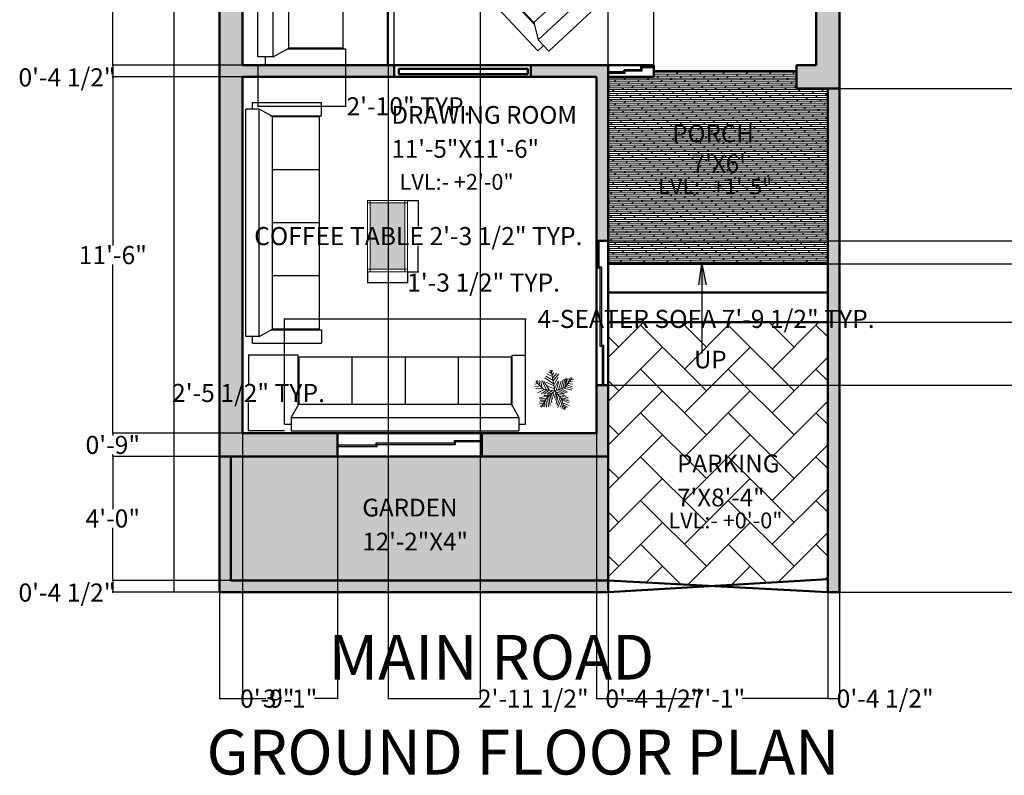
# Model space of a CAD drawing. Units: inches. Extents: x 48 to 822, y -191 to 651.
# Tile 1 of 13: x 48 to 429, y -191 to 101. Entities that reach past the tile are written whole.
import ezdxf

# ---------------------------------------------------------------- set-up
doc = ezdxf.new("R2010")
doc.units = ezdxf.units.IN
doc.header["$MEASUREMENT"] = 0
doc.layers.get('0').update_dxf_attribs({"color": 254})
for name, color, linetype, lineweight in [('A-ANNO-DIMS', 2, 'Continuous', 18), ('A-ANNO-SYMB', 3, 'Continuous', 18), ('A-ANNO-TEXT', 3, 'Continuous', 25), ('A-AREA-IDEN', 7, 'Continuous', 25), ('A-FLOR-PATT', 252, 'Continuous', 13), ('A-FLOR-STRS', 3, 'Continuous', 25), ('A-FURN', 8, 'Continuous', 18), ('A-GLAZ', 4, 'Continuous', 25), ('A-WALL', 7, 'Continuous', 50), ('A-WALL-PATT', 8, 'Continuous', 13), ('L-PLNT', 103, 'Continuous', 18)]:
    doc.layers.add(name, color=color, linetype=linetype, lineweight=lineweight)
doc.layers.add('furniture', color=250, linetype='Continuous')
doc.styles.get("Standard").update_dxf_attribs({"font": 'arial.ttf'})
doc.dimstyles.get("Standard").update_dxf_attribs({"dimtxt": 7, "dimasz": 0.18, "dimexe": 0.18, "dimexo": 0.0625, "dimgap": 0.09, "dimtad": 0, "dimtih": 1, "dimtoh": 1, "dimzin": 0, "dimdsep": 46, "dimlunit": 3, "dimtxsty": 'Standard', "dimcen": 0.09, "dimadec": 0, "dimazin": 0, "dimtfac": 1, "dimtofl": 0, "dimtmove": 0, "dimatfit": 3, "dimfxl": 1, "dimtolj": 1, "dimtzin": 0, "dimarcsym": 0})

# ---------------------------------------------------------------- blocks, each defined once
blk = doc.blocks.new('FABRIC SOFA 1S')
at = {"layer": 'furniture'}
for p, q in [((3, 18.12), (34, 18.12)), ((3, 15.12), (3, 18.12)), ((34, 12.12), (34, 18.12)), ((0, -15.12), (0, 15.12)), ((6, 15.12), (0, 15.12)), ((6, -15.12), (6, 15.12)), ((12, 11.75), (6, 15.12)), ((11.33, 12.12), (34, 12.12)), ((6, -15.12), (0, -15.12)), ((3, -18.12), (3, -15.12)), ((6, -15.12), (12, -11.75)), ((11.33, -12.12), (34, -12.12)), ((34, -12.12), (34, -18.12)), ((3, -18.12), (34, -18.12))]:
    blk.add_line(p, q, dxfattribs=at)
blk.add_lwpolyline([(12, -11.75), (12, 11.75), (33, 11.75), (33, -11.75)], close=True, dxfattribs=at)
blk = doc.blocks.new('FABRIC SOFA 4S')
at = {"layer": 'furniture'}
for p, q in [((3, 54), (34, 54)), ((3, 51), (3, 54)), ((34, 48), (34, 54)), ((0, -51), (0, 51)), ((6, 51), (0, 51)), ((6, -51), (6, 51)), ((12, 47.63), (6, 51)), ((11.14, 48), (34, 48)), ((33, 23.81), (12, 23.81)), ((33, 0), (12, 0)), ((33, -23.81), (12, -23.81)), ((6, -51), (12, -47.63)), ((11.54, -48), (34, -48)), ((34, -48), (34, -54)), ((6, -51), (0, -51)), ((3, -54), (3, -51)), ((3, -54), (34, -54))]:
    blk.add_line(p, q, dxfattribs=at)
blk.add_lwpolyline([(12, -47.63), (12, 47.63), (33, 47.63), (33, -47.63)], close=True, dxfattribs=at)
blk = doc.blocks.new('*U15')
for p, q in [((-10.186, 53.64), (-13.084, 55.962)), ((0, 0), (-10.5, 57)), ((-9.099, 51.782), (-6.563, 55.962)), ((-48.585, 21.131), (-49.309, 29.026)), ((-43.513, 28.561), (-42.427, 15.558)), ((-35.544, 28.097), (-24.314, 3.947)), ((-3.665, 19.273), (-27.574, 35.527)), ((-5.114, 28.097), (-24.676, 40.636)), ((-7.288, 39.707), (-21.778, 46.673)), ((-8.737, 47.138), (-17.069, 52.711)), ((-7.65, 43.423), (-2.578, 49.46)), ((-5.839, 35.992), (4.667, 48.067)), ((-5.114, 27.632), (10.463, 46.673)), ((-2.941, 16.486), (8.652, 37.85)), ((16.259, 5.805), (23.142, 31.348)), ((22.055, 7.198), (27.489, 32.277)), ((27, 9), (48, 36)), ((27.127, 9.056), (31.112, 35.992)), ((31.836, 30.883), (32.561, 16.486)), ((35.096, 32.741), (37.27, 22.524)), ((38.719, 34.134), (41.979, 28.561)), ((43.791, 29.954), (51.036, 30.883)), ((44.153, 36.456), (45.239, 32.741)), ((-47.498, 19.737), (-55.83, 18.344)), ((-40.615, 13.7), (-55.105, 10.913)), ((-31.5, 4.5), (-52.5, 25.5)), ((-33.37, 6.269), (-52.207, 5.34)), ((-28.299, 3.483), (-47.86, -5.805)), ((-38.442, 26.239), (-34.819, 7.663)), ((-21.416, 3.018), (-38.079, -8.128)), ((0, 0), (-31.5, 4.5)), ((-14.533, 2.09), (-30.834, 25.31)), ((-15.982, 2.09), (-30.11, -9.521)), ((-24.314, 23.917), (-2.941, 13.7)), ((0, 0), (-22.5, -19.5)), ((-6.563, 1.161), (-21.416, -8.128)), ((-20.691, 13.7), (-1.129, 4.876)), ((-1.129, 6.734), (9.014, 26.704)), ((0, 0), (27, 9)), ((0, 0), (18, -22.5)), ((3.942, 1.625), (11.187, 24.381)), ((6.478, 1.625), (26.04, -8.592)), ((10.101, 3.483), (17.708, 26.239)), ((11.187, 3.483), (30.749, -5.805)), ((18.07, 5.805), (35.096, -3.483)), ((24.229, 7.663), (46.688, 1.625)), ((29.662, 12.307), (48.137, 6.269)), ((33.285, 16.486), (48.862, 10.913)), ((36.183, 19.737), (48.137, 17.88)), ((40.53, 25.775), (48.862, 24.846)), ((-17.431, -15.094), (-42.789, -18.809)), ((-24.314, -21.596), (-42.427, -22.06)), ((-26.849, -26.24), (-40.253, -25.775)), ((-22.5, -19.5), (-37.5, -45)), ((-15.257, -12.772), (-30.11, -12.772)), ((-25.038, -23.918), (-22.865, -45.281)), ((-20.691, -18.345), (-17.793, -44.352)), ((-6.563, -5.805), (-19.967, -9.985)), ((-17.069, -15.094), (-12.721, -40.172)), ((-13.446, -11.378), (-8.737, -32.741)), ((-9.461, -8.592), (-6.201, -23.453)), ((-4.752, -3.483), (-3.665, -14.629)), ((2.493, -3.019), (-1.491, -20.202)), ((1.769, -2.555), (24.229, -9.521)), ((5.029, -6.27), (2.131, -25.775)), ((9.014, -11.378), (3.58, -35.992)), ((14.085, -16.951), (6.478, -40.172)), ((7.565, -9.056), (32.198, -14.629)), ((18.07, -22.524), (8.289, -45.745)), ((12.274, -15.094), (36.907, -18.809)), ((16.259, -19.738), (36.183, -22.989)), ((18, -22.5), (27, -52.5)), ((18.433, -22.524), (40.53, -29.026)), ((19.157, -25.311), (38.719, -33.206)), ((-28.299, -29.026), (-42.789, -31.348)), ((-30.834, -34.135), (-42.427, -35.528)), ((-34.457, -39.708), (-40.978, -42.494)), ((-32.646, -36.921), (-31.921, -44.352)), ((-29.023, -30.884), (-27.936, -43.887)), ((20.244, -30.419), (15.897, -44.816)), ((22.78, -37.85), (19.519, -48.532)), ((21.331, -32.741), (39.081, -40.636)), ((22.78, -38.314), (34.372, -44.816)), ((24.591, -45.745), (23.142, -50.854)), ((24.591, -43.423), (30.749, -47.603)), ((26.764, -49.925), (28.213, -50.854))]:
    blk.add_line(p, q)
blk = doc.blocks.new('*D17')
at = {"layer": 'A-ANNO-DIMS', "color": 0, "lineweight": -2, "transparency": 16777216}
for p, q in [((109.06, 599.69), (107.79, 599.69)), ((107.97, 599.51), (107.97, 243.35)), ((107.97, -120.13), (107.97, 236.02)), ((109.06, -120.31), (107.79, -120.31))]:
    blk.add_line(p, q, dxfattribs=at)
at = {"layer": 'A-ANNO-DIMS', "color": 0, "transparency": 16777216}
for points in [[(107.94, 599.51), (108, 599.51), (107.97, 599.69)], [(107.94, -120.13), (108, -120.13), (107.97, -120.31)]]:
    blk.add_solid(points, dxfattribs=at)
at = {"layer": 'Defpoints', "color": 0, "transparency": 16777216}
for p in [(109.12, 599.69), (107.97, -120.31), (109.12, -120.31)]:
    blk.add_point(p, dxfattribs=at)
at = {"layer": 'A-ANNO-DIMS', "color": 0, "transparency": 16777216, "insert": (107.97, 239.69), "char_height": 7, "attachment_point": 5}
blk.add_mtext("\\A1;60'", dxfattribs=at)
blk = doc.blocks.new('WIN-1500')
for p, q in [((300.62, 546.44), (315.51, 546.44)), ((300.62, 545.8), (315.95, 545.8)), ((315.51, 546.44), (315.51, 547.24)), ((315.51, 547.24), (345.84, 547.24)), ((315.95, 545.8), (315.95, 546.59)), ((315.95, 546.59), (346.31, 546.59)), ((345.84, 547.24), (345.84, 548.17)), ((345.84, 548.17), (356.45, 548.17)), ((346.31, 546.59), (346.31, 547.73)), ((346.31, 547.73), (356.45, 547.73))]:
    blk.add_line(p, q)
blk = doc.blocks.new('WIN-450')
for p, q in [((145.74, 373.13), (145.74, 373.99)), ((145.74, 373.99), (152.3, 373.99)), ((152.3, 373.99), (152.3, 375.35)), ((152.3, 375.35), (156.91, 375.35)), ((139.16, 373.13), (145.74, 373.13))]:
    blk.add_line(p, q)
blk = doc.blocks.new('COFFEE-TABLE')
for p, q in [((0, 27.69), (0, 0)), ((15.53, 27.69), (0, 27.69)), ((15.53, 0), (15.53, 27.69)), ((0, 0), (15.53, 0))]:
    blk.add_line(p, q)
blk = doc.blocks.new('*D30')
at = {"layer": 'A-ANNO-DIMS', "color": 0, "lineweight": -2, "transparency": 16777216}
for p, q in [((174.35, 192), (190.67, 192)), ((190.49, 191.82), (190.49, 141.72)), ((190.49, 84.18), (190.49, 134.29)), ((174.35, 84), (190.67, 84))]:
    blk.add_line(p, q, dxfattribs=at)
at = {"layer": 'A-ANNO-DIMS', "color": 0, "transparency": 16777216}
for points in [[(190.46, 191.82), (190.52, 191.82), (190.49, 192)], [(190.46, 84.18), (190.52, 84.18), (190.49, 84)]]:
    blk.add_solid(points, dxfattribs=at)
at = {"layer": 'Defpoints', "color": 0, "transparency": 16777216}
for p in [(174.29, 192), (190.49, 192), (174.29, 84)]:
    blk.add_point(p, dxfattribs=at)
at = {"layer": 'A-ANNO-DIMS', "color": 0, "transparency": 16777216, "insert": (190.49, 138), "char_height": 7, "attachment_point": 5}
blk.add_mtext('\\A1;4-SEATER SOFA 9\'-0" TYP.', dxfattribs=at)
blk = doc.blocks.new('*D31')
at = {"layer": 'A-ANNO-DIMS', "color": 0, "lineweight": -2, "transparency": 16777216}
for p, q in [((140.29, 83.94), (140.29, 67.62)), ((174.29, 83.94), (174.29, 67.62)), ((140.47, 67.8), (174.11, 67.8)), ((174.29, 67.8), (174.47, 67.8))]:
    blk.add_line(p, q, dxfattribs=at)
at = {"layer": 'A-ANNO-DIMS', "color": 0, "transparency": 16777216}
for points in [[(140.47, 67.83), (140.47, 67.77), (140.29, 67.8)], [(174.11, 67.83), (174.11, 67.77), (174.29, 67.8)]]:
    blk.add_solid(points, dxfattribs=at)
at = {"layer": 'Defpoints', "color": 0, "transparency": 16777216}
for p in [(140.29, 84), (174.29, 84), (174.29, 67.8)]:
    blk.add_point(p, dxfattribs=at)
at = {"layer": 'A-ANNO-DIMS', "color": 0, "transparency": 16777216, "insert": (198.67, 67.8), "char_height": 7, "attachment_point": 5}
blk.add_mtext('\\A1;2\'-10" TYP.', dxfattribs=at)
blk = doc.blocks.new('*D32')
at = {"layer": 'A-ANNO-DIMS', "color": 0, "lineweight": -2, "transparency": 16777216}
for p, q in [((150.71, -28.45), (150.71, -14.34)), ((150.89, -14.52), (243.82, -14.52)), ((244, -28.45), (244, -14.34)), ((244, -14.52), (244.18, -14.52))]:
    blk.add_line(p, q, dxfattribs=at)
at = {"layer": 'A-ANNO-DIMS', "color": 0, "transparency": 16777216}
for points in [[(150.89, -14.49), (150.89, -14.55), (150.71, -14.52)], [(243.82, -14.49), (243.82, -14.55), (244, -14.52)]]:
    blk.add_solid(points, dxfattribs=at)
at = {"layer": 'Defpoints', "color": 0, "transparency": 16777216}
for p in [(244, -14.52), (150.71, -28.52), (244, -28.52)]:
    blk.add_point(p, dxfattribs=at)
at = {"layer": 'A-ANNO-DIMS', "color": 0, "transparency": 16777216, "insert": (313.84, -14.52), "char_height": 7, "attachment_point": 5}
blk.add_mtext('\\A1;4-SEATER SOFA 7\'-9 1/2" TYP.', dxfattribs=at)
blk = doc.blocks.new('*D33')
at = {"layer": 'A-ANNO-DIMS', "color": 0, "lineweight": -2, "transparency": 16777216}
for p, q in [((150.65, -28.52), (136.54, -28.52)), ((136.72, -28.7), (136.72, -39.49)), ((136.72, -57.7), (136.72, -46.91)), ((150.65, -57.88), (136.54, -57.88))]:
    blk.add_line(p, q, dxfattribs=at)
at = {"layer": 'A-ANNO-DIMS', "color": 0, "transparency": 16777216}
for points in [[(136.69, -28.7), (136.75, -28.7), (136.72, -28.52)], [(136.69, -57.7), (136.75, -57.7), (136.72, -57.88)]]:
    blk.add_solid(points, dxfattribs=at)
at = {"layer": 'Defpoints', "color": 0, "transparency": 16777216}
for p in [(136.72, -28.52), (150.71, -28.52), (150.71, -57.88)]:
    blk.add_point(p, dxfattribs=at)
at = {"layer": 'A-ANNO-DIMS', "color": 0, "transparency": 16777216, "insert": (136.72, -43.2), "char_height": 7, "attachment_point": 5}
blk.add_mtext('\\A1;2\'-5 1/2" TYP.', dxfattribs=at)
blk = doc.blocks.new('*D44')
at = {"layer": 'A-ANNO-DIMS', "color": 0, "lineweight": -2, "transparency": 16777216}
for p, q in [((250.22, 140.52), (223.98, 116.03)), ((254.02, 136.71), (250.22, 140.77)), ((223.72, 115.78), (223.54, 115.78)), ((223.85, 115.9), (223.72, 115.78)), ((227.52, 111.97), (223.73, 116.03))]:
    blk.add_line(p, q, dxfattribs=at)
at = {"layer": 'A-ANNO-DIMS', "color": 0, "transparency": 16777216}
for points in [[(250.2, 140.54), (250.24, 140.49), (250.35, 140.64)], [(223.96, 116.05), (224, 116), (223.85, 115.9)]]:
    blk.add_solid(points, dxfattribs=at)
at = {"layer": 'Defpoints', "color": 0, "transparency": 16777216}
for p in [(254.06, 136.66), (223.85, 115.9), (227.56, 111.93)]:
    blk.add_point(p, dxfattribs=at)
at = {"layer": 'A-ANNO-DIMS', "color": 0, "transparency": 16777216, "insert": (174.76, 115.78), "char_height": 7, "attachment_point": 5}
blk.add_mtext('\\A1;SOFA CHAIR 3\'-0 1/2"', dxfattribs=at)
blk = doc.blocks.new('*D48')
at = {"layer": 'A-ANNO-DIMS', "color": 0, "lineweight": -2, "transparency": 16777216}
for p, q in [((198.36, 31.39), (202.63, 31.39)), ((202.45, 31.21), (202.45, 21.26)), ((202.45, 3.88), (202.45, 13.83)), ((198.36, 3.7), (202.63, 3.7))]:
    blk.add_line(p, q, dxfattribs=at)
at = {"layer": 'A-ANNO-DIMS', "color": 0, "transparency": 16777216}
for points in [[(202.42, 31.21), (202.48, 31.21), (202.45, 31.39)], [(202.42, 3.88), (202.48, 3.88), (202.45, 3.7)]]:
    blk.add_solid(points, dxfattribs=at)
at = {"layer": 'Defpoints', "color": 0, "transparency": 16777216}
for p in [(198.3, 31.39), (202.45, 31.39), (198.3, 3.7)]:
    blk.add_point(p, dxfattribs=at)
at = {"layer": 'A-ANNO-DIMS', "color": 0, "transparency": 16777216, "insert": (202.45, 17.55), "char_height": 7, "attachment_point": 5}
blk.add_mtext('\\A1;COFFEE TABLE 2\'-3 1/2" TYP.', dxfattribs=at)
blk = doc.blocks.new('*D49')
at = {"layer": 'A-ANNO-DIMS', "color": 0, "lineweight": -2, "transparency": 16777216}
for p, q in [((182.77, 3.64), (182.77, -0.63)), ((198.3, 3.64), (198.3, -0.63)), ((182.95, -0.45), (198.12, -0.45)), ((198.3, -0.45), (198.48, -0.45))]:
    blk.add_line(p, q, dxfattribs=at)
at = {"layer": 'A-ANNO-DIMS', "color": 0, "transparency": 16777216}
for points in [[(182.95, -0.42), (182.95, -0.48), (182.77, -0.45)], [(198.12, -0.42), (198.12, -0.48), (198.3, -0.45)]]:
    blk.add_solid(points, dxfattribs=at)
at = {"layer": 'Defpoints', "color": 0, "transparency": 16777216}
for p in [(182.77, 3.7), (198.3, 3.7), (198.3, -0.45)]:
    blk.add_point(p, dxfattribs=at)
at = {"layer": 'A-ANNO-DIMS', "color": 0, "transparency": 16777216, "insert": (227.73, -0.45), "char_height": 7, "attachment_point": 5}
blk.add_mtext('\\A1;1\'-3 1/2" TYP.', dxfattribs=at)
blk = doc.blocks.new('*D65')
at = {"layer": 'A-ANNO-DIMS', "color": 0, "lineweight": -2, "transparency": 16777216}
for p, q in [((134.45, -58.88), (134.45, -161.74)), ((125.45, -120.38), (125.45, -161.74)), ((125.63, -161.56), (134.27, -161.56)), ((134.45, -161.56), (134.63, -161.56))]:
    blk.add_line(p, q, dxfattribs=at)
at = {"layer": 'A-ANNO-DIMS', "color": 0, "transparency": 16777216}
for points in [[(125.63, -161.53), (125.63, -161.59), (125.45, -161.56)], [(134.27, -161.53), (134.27, -161.59), (134.45, -161.56)]]:
    blk.add_solid(points, dxfattribs=at)
at = {"layer": 'Defpoints', "color": 0, "transparency": 16777216}
for p in [(134.45, -58.81), (125.45, -120.31), (134.45, -161.56)]:
    blk.add_point(p, dxfattribs=at)
at = {"layer": 'A-ANNO-DIMS', "color": 0, "transparency": 16777216, "insert": (144.02, -161.56), "char_height": 7, "attachment_point": 5}
blk.add_mtext('\\A1;0\'-9"', dxfattribs=at)
blk = doc.blocks.new('*D66')
at = {"layer": 'A-ANNO-DIMS', "color": 0, "lineweight": -2, "transparency": 16777216}
for p, q in [((271.45, -58.88), (271.45, -161.74)), ((275.95, -120.38), (275.95, -161.74)), ((271.63, -161.56), (275.77, -161.56)), ((275.95, -161.56), (276.13, -161.56))]:
    blk.add_line(p, q, dxfattribs=at)
at = {"layer": 'A-ANNO-DIMS', "color": 0, "transparency": 16777216}
for points in [[(271.63, -161.53), (271.63, -161.59), (271.45, -161.56)], [(275.77, -161.53), (275.77, -161.59), (275.95, -161.56)]]:
    blk.add_solid(points, dxfattribs=at)
at = {"layer": 'Defpoints', "color": 0, "transparency": 16777216}
for p in [(271.45, -58.81), (275.95, -120.31), (275.95, -161.56)]:
    blk.add_point(p, dxfattribs=at)
at = {"layer": 'A-ANNO-DIMS', "color": 0, "transparency": 16777216, "insert": (293.68, -161.56), "char_height": 7, "attachment_point": 5}
blk.add_mtext('\\A1;0\'-4 1/2"', dxfattribs=at)
blk = doc.blocks.new('*D67')
at = {"layer": 'A-ANNO-DIMS', "color": 0, "lineweight": -2, "transparency": 16777216}
for p, q in [((275.95, -120.38), (275.95, -161.74)), ((360.95, -120.38), (360.95, -161.74)), ((276.13, -161.56), (309.09, -161.56)), ((360.77, -161.56), (327.82, -161.56))]:
    blk.add_line(p, q, dxfattribs=at)
at = {"layer": 'A-ANNO-DIMS', "color": 0, "transparency": 16777216}
for points in [[(276.13, -161.53), (276.13, -161.59), (275.95, -161.56)], [(360.77, -161.53), (360.77, -161.59), (360.95, -161.56)]]:
    blk.add_solid(points, dxfattribs=at)
at = {"layer": 'Defpoints', "color": 0, "transparency": 16777216}
for p in [(275.95, -120.31), (360.95, -120.31), (360.95, -161.56)]:
    blk.add_point(p, dxfattribs=at)
at = {"layer": 'A-ANNO-DIMS', "color": 0, "transparency": 16777216, "insert": (318.45, -161.56), "char_height": 7, "attachment_point": 5}
blk.add_mtext('\\A1;7\'-1"', dxfattribs=at)
blk = doc.blocks.new('*D68')
at = {"layer": 'A-ANNO-DIMS', "color": 0, "lineweight": -2, "transparency": 16777216}
for p, q in [((360.95, -120.38), (360.95, -161.74)), ((365.45, -120.38), (365.45, -161.74)), ((361.13, -161.56), (365.27, -161.56)), ((365.45, -161.56), (365.63, -161.56))]:
    blk.add_line(p, q, dxfattribs=at)
at = {"layer": 'A-ANNO-DIMS', "color": 0, "transparency": 16777216}
for points in [[(361.13, -161.53), (361.13, -161.59), (360.95, -161.56)], [(365.27, -161.53), (365.27, -161.59), (365.45, -161.56)]]:
    blk.add_solid(points, dxfattribs=at)
at = {"layer": 'Defpoints', "color": 0, "transparency": 16777216}
for p in [(360.95, -120.31), (365.45, -120.31), (365.45, -161.56)]:
    blk.add_point(p, dxfattribs=at)
at = {"layer": 'A-ANNO-DIMS', "color": 0, "transparency": 16777216, "insert": (383.18, -161.56), "char_height": 7, "attachment_point": 5}
blk.add_mtext('\\A1;0\'-4 1/2"', dxfattribs=at)
blk = doc.blocks.new('*D69')
at = {"layer": 'A-ANNO-DIMS', "color": 0, "lineweight": -2, "transparency": 16777216}
for p, q in [((134.45, -58.88), (134.45, -161.74)), ((171.2, -58.88), (171.2, -161.74)), ((134.63, -161.56), (143.44, -161.56)), ((171.02, -161.56), (162.22, -161.56))]:
    blk.add_line(p, q, dxfattribs=at)
at = {"layer": 'A-ANNO-DIMS', "color": 0, "transparency": 16777216}
for points in [[(134.63, -161.53), (134.63, -161.59), (134.45, -161.56)], [(171.02, -161.53), (171.02, -161.59), (171.2, -161.56)]]:
    blk.add_solid(points, dxfattribs=at)
at = {"layer": 'Defpoints', "color": 0, "transparency": 16777216}
for p in [(134.45, -58.81), (171.2, -58.81), (171.2, -161.56)]:
    blk.add_point(p, dxfattribs=at)
at = {"layer": 'A-ANNO-DIMS', "color": 0, "transparency": 16777216, "insert": (152.83, -161.56), "char_height": 7, "attachment_point": 5}
blk.add_mtext('\\A1;3\'-1"', dxfattribs=at)
blk = doc.blocks.new('*D78')
at = {"layer": 'A-ANNO-DIMS', "color": 0, "lineweight": -2, "transparency": 16777216}
for p, q in [((134.39, 221.69), (84.02, 221.69)), ((84.2, 221.51), (84.2, 156.35)), ((84.2, 83.87), (84.2, 149.02)), ((134.39, 83.69), (84.02, 83.69))]:
    blk.add_line(p, q, dxfattribs=at)
at = {"layer": 'A-ANNO-DIMS', "color": 0, "transparency": 16777216}
for points in [[(84.17, 221.51), (84.23, 221.51), (84.2, 221.69)], [(84.17, 83.87), (84.23, 83.87), (84.2, 83.69)]]:
    blk.add_solid(points, dxfattribs=at)
at = {"layer": 'Defpoints', "color": 0, "transparency": 16777216}
for p in [(134.45, 221.69), (84.2, 83.69), (134.45, 83.69)]:
    blk.add_point(p, dxfattribs=at)
at = {"layer": 'A-ANNO-DIMS', "color": 0, "transparency": 16777216, "insert": (84.2, 152.69), "char_height": 7, "attachment_point": 5}
blk.add_mtext('\\A1;11\'-6"', dxfattribs=at)
blk = doc.blocks.new('*D79')
at = {"layer": 'A-ANNO-DIMS', "color": 0, "lineweight": -2, "transparency": 16777216}
for p, q in [((134.39, 83.69), (84.02, 83.69)), ((84.2, 83.51), (84.2, 79.37)), ((134.39, 79.19), (84.02, 79.19)), ((84.2, 79.01), (84.02, 79.01)), ((84.2, 79.19), (84.2, 79.01))]:
    blk.add_line(p, q, dxfattribs=at)
at = {"layer": 'A-ANNO-DIMS', "color": 0, "transparency": 16777216}
for points in [[(84.17, 83.51), (84.23, 83.51), (84.2, 83.69)], [(84.17, 79.37), (84.23, 79.37), (84.2, 79.19)]]:
    blk.add_solid(points, dxfattribs=at)
at = {"layer": 'Defpoints', "color": 0, "transparency": 16777216}
for p in [(134.45, 83.69), (84.2, 79.19), (134.45, 79.19)]:
    blk.add_point(p, dxfattribs=at)
at = {"layer": 'A-ANNO-DIMS', "color": 0, "transparency": 16777216, "insert": (66.47, 79.01), "char_height": 7, "attachment_point": 5}
blk.add_mtext('\\A1;0\'-4 1/2"', dxfattribs=at)
blk = doc.blocks.new('*D80')
at = {"layer": 'A-ANNO-DIMS', "color": 0, "lineweight": -2, "transparency": 16777216}
for p, q in [((134.39, 79.19), (84.02, 79.19)), ((84.2, 79.01), (84.2, 13.85)), ((84.2, -58.63), (84.2, 6.52)), ((134.39, -58.81), (84.02, -58.81))]:
    blk.add_line(p, q, dxfattribs=at)
at = {"layer": 'A-ANNO-DIMS', "color": 0, "transparency": 16777216}
for points in [[(84.17, 79.01), (84.23, 79.01), (84.2, 79.19)], [(84.17, -58.63), (84.23, -58.63), (84.2, -58.81)]]:
    blk.add_solid(points, dxfattribs=at)
at = {"layer": 'Defpoints', "color": 0, "transparency": 16777216}
for p in [(134.45, 79.19), (84.2, -58.81), (134.45, -58.81)]:
    blk.add_point(p, dxfattribs=at)
at = {"layer": 'A-ANNO-DIMS', "color": 0, "transparency": 16777216, "insert": (84.2, 10.19), "char_height": 7, "attachment_point": 5}
blk.add_mtext('\\A1;11\'-6"', dxfattribs=at)
blk = doc.blocks.new('*D81')
at = {"layer": 'A-ANNO-DIMS', "color": 0, "lineweight": -2, "transparency": 16777216}
for p, q in [((134.39, -58.81), (84.02, -58.81)), ((84.2, -58.99), (84.2, -59.65)), ((129.89, -67.81), (84.02, -67.81)), ((84.2, -67.63), (84.2, -66.98))]:
    blk.add_line(p, q, dxfattribs=at)
at = {"layer": 'A-ANNO-DIMS', "color": 0, "transparency": 16777216}
for points in [[(84.17, -58.99), (84.23, -58.99), (84.2, -58.81)], [(84.17, -67.63), (84.23, -67.63), (84.2, -67.81)]]:
    blk.add_solid(points, dxfattribs=at)
at = {"layer": 'Defpoints', "color": 0, "transparency": 16777216}
for p in [(134.45, -58.81), (84.2, -67.81), (129.95, -67.81)]:
    blk.add_point(p, dxfattribs=at)
at = {"layer": 'A-ANNO-DIMS', "color": 0, "transparency": 16777216, "insert": (84.2, -63.31), "char_height": 7, "attachment_point": 5}
blk.add_mtext('\\A1;0\'-9"', dxfattribs=at)
blk = doc.blocks.new('*D82')
at = {"layer": 'A-ANNO-DIMS', "color": 0, "lineweight": -2, "transparency": 16777216}
for p, q in [((129.89, -67.81), (84.02, -67.81)), ((84.2, -67.99), (84.2, -88.15)), ((84.2, -115.63), (84.2, -95.48)), ((129.89, -115.81), (84.02, -115.81))]:
    blk.add_line(p, q, dxfattribs=at)
at = {"layer": 'A-ANNO-DIMS', "color": 0, "transparency": 16777216}
for points in [[(84.17, -67.99), (84.23, -67.99), (84.2, -67.81)], [(84.17, -115.63), (84.23, -115.63), (84.2, -115.81)]]:
    blk.add_solid(points, dxfattribs=at)
at = {"layer": 'Defpoints', "color": 0, "transparency": 16777216}
for p in [(129.95, -67.81), (84.2, -115.81), (129.95, -115.81)]:
    blk.add_point(p, dxfattribs=at)
at = {"layer": 'A-ANNO-DIMS', "color": 0, "transparency": 16777216, "insert": (84.2, -91.81), "char_height": 7, "attachment_point": 5}
blk.add_mtext('\\A1;4\'-0"', dxfattribs=at)
blk = doc.blocks.new('*D83')
at = {"layer": 'A-ANNO-DIMS', "color": 0, "lineweight": -2, "transparency": 16777216}
for p, q in [((129.89, -115.81), (84.02, -115.81)), ((84.2, -115.99), (84.2, -120.13)), ((125.39, -120.31), (84.02, -120.31)), ((84.2, -120.49), (84.02, -120.49)), ((84.2, -120.31), (84.2, -120.49))]:
    blk.add_line(p, q, dxfattribs=at)
at = {"layer": 'A-ANNO-DIMS', "color": 0, "transparency": 16777216}
for points in [[(84.17, -115.99), (84.23, -115.99), (84.2, -115.81)], [(84.17, -120.13), (84.23, -120.13), (84.2, -120.31)]]:
    blk.add_solid(points, dxfattribs=at)
at = {"layer": 'Defpoints', "color": 0, "transparency": 16777216}
for p in [(129.95, -115.81), (84.2, -120.31), (125.45, -120.31)]:
    blk.add_point(p, dxfattribs=at)
at = {"layer": 'A-ANNO-DIMS', "color": 0, "transparency": 16777216, "insert": (66.47, -120.49), "char_height": 7, "attachment_point": 5}
blk.add_mtext('\\A1;0\'-4 1/2"', dxfattribs=at)
blk = doc.blocks.new('*D86')
at = {"layer": 'A-ANNO-DIMS', "color": 0, "lineweight": -2, "transparency": 16777216}
for p, q in [((361.01, 74.69), (790.04, 74.69)), ((789.86, 74.51), (789.86, 44.42)), ((789.86, 7.02), (789.86, 37.1)), ((361.01, 6.84), (790.04, 6.84))]:
    blk.add_line(p, q, dxfattribs=at)
at = {"layer": 'A-ANNO-DIMS', "color": 0, "transparency": 16777216}
for points in [[(789.83, 74.51), (789.89, 74.51), (789.86, 74.69)], [(789.83, 7.02), (789.89, 7.02), (789.86, 6.84)]]:
    blk.add_solid(points, dxfattribs=at)
at = {"layer": 'Defpoints', "color": 0, "transparency": 16777216}
for p in [(360.95, 74.69), (360.95, 6.84), (789.86, 6.84)]:
    blk.add_point(p, dxfattribs=at)
at = {"layer": 'A-ANNO-DIMS', "color": 0, "transparency": 16777216, "insert": (789.86, 40.76), "char_height": 7, "attachment_point": 5}
blk.add_mtext('\\A1;5\'-8"', dxfattribs=at)
blk = doc.blocks.new('*D87')
at = {"layer": 'A-ANNO-DIMS', "color": 0, "lineweight": -2, "transparency": 16777216}
for p, q in [((361.01, 6.84), (790.04, 6.84)), ((789.86, 6.66), (789.86, -0.78)), ((789.86, -15.63), (789.86, -8.2)), ((361.01, -15.81), (790.04, -15.81))]:
    blk.add_line(p, q, dxfattribs=at)
at = {"layer": 'A-ANNO-DIMS', "color": 0, "transparency": 16777216}
for points in [[(789.83, 6.66), (789.89, 6.66), (789.86, 6.84)], [(789.83, -15.63), (789.89, -15.63), (789.86, -15.81)]]:
    blk.add_solid(points, dxfattribs=at)
at = {"layer": 'Defpoints', "color": 0, "transparency": 16777216}
for p in [(360.95, 6.84), (360.95, -15.81), (789.86, -15.81)]:
    blk.add_point(p, dxfattribs=at)
at = {"layer": 'A-ANNO-DIMS', "color": 0, "transparency": 16777216, "insert": (789.86, -4.49), "char_height": 7, "attachment_point": 5}
blk.add_mtext('\\A1;1\'-10 1/2"', dxfattribs=at)
blk = doc.blocks.new('*D88')
at = {"layer": 'A-ANNO-DIMS', "color": 0, "lineweight": -2, "transparency": 16777216}
for p, q in [((361.01, -15.81), (790.04, -15.81)), ((789.86, -15.99), (789.86, -64.35)), ((789.86, -120.13), (789.86, -71.77)), ((365.51, -120.31), (790.04, -120.31))]:
    blk.add_line(p, q, dxfattribs=at)
at = {"layer": 'A-ANNO-DIMS', "color": 0, "transparency": 16777216}
for points in [[(789.83, -15.99), (789.89, -15.99), (789.86, -15.81)], [(789.83, -120.13), (789.89, -120.13), (789.86, -120.31)]]:
    blk.add_solid(points, dxfattribs=at)
at = {"layer": 'Defpoints', "color": 0, "transparency": 16777216}
for p in [(360.95, -15.81), (365.45, -120.31), (789.86, -120.31)]:
    blk.add_point(p, dxfattribs=at)
at = {"layer": 'A-ANNO-DIMS', "color": 0, "transparency": 16777216, "insert": (789.86, -68.06), "char_height": 7, "attachment_point": 5}
blk.add_mtext('\\A1;8\'-8 1/2"', dxfattribs=at)
blk = doc.blocks.new('*D92')
at = {"layer": 'A-ANNO-DIMS', "color": 0, "lineweight": -2, "transparency": 16777216}
for p, q in [((275.91, 79.24), (275.91, 641.12)), ((276.09, 640.94), (293.48, 640.94)), ((293.66, 79.24), (293.66, 641.12)), ((293.66, 640.94), (293.84, 640.94))]:
    blk.add_line(p, q, dxfattribs=at)
at = {"layer": 'A-ANNO-DIMS', "color": 0, "transparency": 16777216}
for points in [[(276.09, 640.97), (276.09, 640.91), (275.91, 640.94)], [(293.48, 640.97), (293.48, 640.91), (293.66, 640.94)]]:
    blk.add_solid(points, dxfattribs=at)
at = {"layer": 'Defpoints', "color": 0, "transparency": 16777216}
for p in [(293.66, 640.94), (275.91, 79.18), (293.66, 79.18)]:
    blk.add_point(p, dxfattribs=at)
at = {"layer": 'A-ANNO-DIMS', "color": 0, "transparency": 16777216, "insert": (302.9, 640.94), "char_height": 7, "attachment_point": 5}
blk.add_mtext('\\A1;1\'-6"', dxfattribs=at)
blk = doc.blocks.new('*D93')
at = {"layer": 'A-ANNO-DIMS', "color": 0, "lineweight": -2, "transparency": 16777216}
for p, q in [((271.51, 15.7), (790.04, 15.7)), ((789.86, 15.52), (789.86, -8.55)), ((789.86, -39.95), (789.86, -15.88)), ((271.51, -40.13), (790.04, -40.13))]:
    blk.add_line(p, q, dxfattribs=at)
at = {"layer": 'A-ANNO-DIMS', "color": 0, "transparency": 16777216}
for points in [[(789.83, 15.52), (789.89, 15.52), (789.86, 15.7)], [(789.83, -39.95), (789.89, -39.95), (789.86, -40.13)]]:
    blk.add_solid(points, dxfattribs=at)
at = {"layer": 'Defpoints', "color": 0, "transparency": 16777216}
for p in [(271.45, 15.7), (271.45, -40.13), (789.86, -40.13)]:
    blk.add_point(p, dxfattribs=at)
at = {"layer": 'A-ANNO-DIMS', "color": 0, "transparency": 16777216, "insert": (789.86, -12.22), "char_height": 7, "attachment_point": 5}
blk.add_mtext('\\A1;4\'-8"', dxfattribs=at)
blk = doc.blocks.new('*D94')
at = {"layer": 'A-ANNO-DIMS', "color": 0, "lineweight": -2, "transparency": 16777216}
for p, q in [((134.45, 83.75), (134.45, 641.12)), ((134.63, 640.94), (143.35, 640.94)), ((192.89, 640.94), (184.17, 640.94)), ((193.07, 83.75), (193.07, 641.12))]:
    blk.add_line(p, q, dxfattribs=at)
at = {"layer": 'A-ANNO-DIMS', "color": 0, "transparency": 16777216}
for points in [[(134.63, 640.97), (134.63, 640.91), (134.45, 640.94)], [(192.89, 640.97), (192.89, 640.91), (193.07, 640.94)]]:
    blk.add_solid(points, dxfattribs=at)
at = {"layer": 'Defpoints', "color": 0, "transparency": 16777216}
for p in [(193.07, 640.94), (134.45, 83.69), (193.07, 83.69)]:
    blk.add_point(p, dxfattribs=at)
at = {"layer": 'A-ANNO-DIMS', "color": 0, "transparency": 16777216, "insert": (163.76, 640.94), "char_height": 7, "attachment_point": 5}
blk.add_mtext('\\A1;4\'-10 1/2"', dxfattribs=at)
blk = doc.blocks.new('*D95')
at = {"layer": 'A-ANNO-DIMS', "color": 0, "lineweight": -2, "transparency": 16777216}
for p, q in [((226.45, 434.62), (226.45, -161.74)), ((190.77, 432.37), (190.77, -161.74)), ((190.95, -161.56), (226.27, -161.56)), ((226.45, -161.56), (226.63, -161.56))]:
    blk.add_line(p, q, dxfattribs=at)
at = {"layer": 'A-ANNO-DIMS', "color": 0, "transparency": 16777216}
for points in [[(190.95, -161.53), (190.95, -161.59), (190.77, -161.56)], [(226.27, -161.53), (226.27, -161.59), (226.45, -161.56)]]:
    blk.add_solid(points, dxfattribs=at)
at = {"layer": 'Defpoints', "color": 0, "transparency": 16777216}
for p in [(226.45, 434.69), (190.77, 432.44), (226.45, -161.56)]:
    blk.add_point(p, dxfattribs=at)
at = {"layer": 'A-ANNO-DIMS', "color": 0, "transparency": 16777216, "insert": (246.96, -161.56), "char_height": 7, "attachment_point": 5}
blk.add_mtext('\\A1;2\'-11 1/2"', dxfattribs=at)

msp = doc.modelspace()

# ---------------------------------------------------------------- hatches: boundary and pattern name
at = {"layer": 'A-ANNO-SYMB'}
h = msp.add_hatch(color=256, dxfattribs=at)
h.dxf.hatch_style = 1
h.paths.add_polyline_path([(313.906, -1.331), (312.262, 6.835), (310.985, -1.331)])
at = {"layer": 'A-FLOR-PATT'}
h = msp.add_hatch(dxfattribs=at)
h.set_pattern_fill('AR-HBONE', color=256, scale=3)
h.paths.add_polyline_path([(360.951, -15.813), (275.951, -15.813), (275.951, -40.13), (275.951, -115.813), (316.207, -117.945), (360.951, -115.312)])
h.paths.add_polyline_path([(307.45, -35.539), (324.172, -35.539), (324.172, -25.123), (307.45, -25.123)], flags=24)
at = {"layer": 'A-FURN'}
h = msp.add_hatch(color=256, dxfattribs=at)
h.dxf.hatch_style = 1
h.paths.add_polyline_path([(197.296, 30.392), (183.771, 30.392), (183.771, 4.7), (197.296, 4.7)])
at = {"layer": 'A-GLAZ'}
h = msp.add_hatch(color=256, dxfattribs=at)
h.dxf.hatch_style = 1
h.paths.add_polyline_path([(282.488, 81.477), (289.048, 81.477), (289.048, 82.837), (293.659, 82.837), (293.659, 83.18), (288.667, 83.18), (288.667, 81.837), (282.184, 81.837), (282.184, 80.962), (275.909, 80.962), (275.909, 80.617), (282.488, 80.617)])
at = {"layer": 'A-WALL-PATT'}
h = msp.add_hatch(color=256, dxfattribs=at)
h.dxf.hatch_style = 1
h.paths.add_polyline_path([(134.451, 590.687), (267.451, 590.687), (267.451, 585.522), (271.951, 585.522), (271.951, 590.687), (356.451, 590.687), (356.451, 83.687), (348.824, 83.687), (348.824, 74.687), (365.451, 74.687), (365.451, 599.687), (125.451, 599.687), (125.451, -67.813), (171.204, -67.813), (171.204, -58.813), (134.451, -58.813), (134.451, 79.187), (193.069, 79.187), (193.069, 83.687), (134.451, 83.687), (134.451, 430.187), (190.775, 430.187), (190.775, 434.687), (134.451, 434.687)])
h.paths.add_polyline_path([(271.951, 550.72), (267.451, 550.72), (267.451, 430.187), (271.951, 430.187)], flags=17)
h.paths.add_polyline_path([(230.951, 432.437), (226.451, 432.437), (226.451, 376.187), (156.909, 376.187), (156.909, 371.687), (164.451, 371.687), (164.451, 359.12), (168.951, 359.12), (168.951, 371.687), (226.451, 371.687), (226.451, 335.687), (230.951, 335.687)], flags=17)
h.paths.add_polyline_path([(168.951, 341.37), (164.451, 341.37), (164.451, 299.687), (134.451, 299.687), (134.451, 295.187), (230.951, 295.187), (230.951, 299.687), (168.951, 299.687)], flags=17)
h.paths.add_polyline_path([(275.909, 83.687), (271.451, 83.687), (245.975, 83.687), (245.975, 79.187), (271.451, 79.187), (271.451, 15.696), (275.951, 15.696), (275.951, 79.177), (275.909, 79.177)], flags=17)
h.paths.add_polyline_path([(275.951, -40.13), (271.451, -40.13), (271.451, -58.813), (227.03, -58.813), (227.03, -67.813), (275.951, -67.813)], flags=17)
h = msp.add_hatch(color=256, dxfattribs=at)
h.dxf.hatch_style = 1
h.paths.add_polyline_path([(365.451, 74.687), (360.951, 74.687), (360.951, -120.313), (365.451, -120.313)])
h.paths.add_polyline_path([(275.951, -115.813), (129.951, -115.813), (129.951, -67.813), (125.451, -67.813), (125.451, -120.313), (275.951, -120.313)])
h.paths.add_polyline_path([(748.61, -21.344), (743.11, -21.344), (743.11, -120.313), (748.61, -120.313)])
h = msp.add_hatch(color=256, dxfattribs=at)
h.dxf.hatch_style = 1
h.paths.add_polyline_path([(216.887, -62.023), (227.03, -62.023), (227.03, -61.583), (216.418, -61.583), (216.418, -62.508), (186.092, -62.508), (186.092, -63.313), (171.204, -63.313), (171.204, -63.954), (186.533, -63.954), (186.533, -63.161), (216.887, -63.161)])
h.paths.add_polyline_path([(588.796, -114.523), (598.94, -114.523), (598.94, -114.083), (588.328, -114.083), (588.328, -115.008), (558.002, -115.008), (558.002, -115.813), (543.114, -115.813), (543.114, -116.454), (558.443, -116.454), (558.443, -115.661), (588.796, -115.661)])
h.paths.add_polyline_path([(656.709, -41.646), (655.571, -41.646), (655.571, -31.502), (655.131, -31.502), (655.131, -42.114), (656.055, -42.114), (656.055, -72.44), (656.86, -72.44), (656.86, -87.328), (657.501, -87.328), (657.501, -72), (656.709, -72)])
h.paths.add_polyline_path([(273.549, 5.552), (272.411, 5.552), (272.411, 15.696), (271.971, 15.696), (271.971, 5.084), (272.896, 5.084), (272.896, -25.242), (273.701, -25.242), (273.701, -40.13), (274.342, -40.13), (274.342, -24.802), (273.549, -24.802)])
at = {"layer": 'L-PLNT'}
h = msp.add_hatch(dxfattribs=at)
h.set_pattern_fill('DOLMIT', color=256, scale=3)
h.paths.add_polyline_path([(360.951, 74.687), (348.824, 74.687), (348.824, 81.427), (293.659, 81.427), (293.659, 79.177), (275.951, 79.177), (275.951, 6.835), (360.951, 6.835)])
h = msp.add_hatch(dxfattribs=at)
h.set_pattern_fill('ESCHER', color=256, scale=3)
h.paths.add_polyline_path([(275.951, -67.813), (129.951, -67.813), (129.951, -115.813), (275.951, -115.813)])

# ---------------------------------------------------------------- linework, layer by layer
at = {"layer": 'A-FLOR-STRS'}
for p, q in [((310.985, -1.331), (312.262, 6.835)), ((312.262, 6.835), (312.262, -27.971)), ((312.262, 6.835), (313.906, -1.331))]:
    msp.add_line(p, q, dxfattribs=at)
at = {"layer": 'A-FURN'}
for p, q in [((183.771, 31.392), (183.771, 3.7)), ((197.296, 3.7), (197.296, 31.392)), ((198.296, 30.392), (182.771, 30.392)), ((182.771, 4.7), (198.296, 4.7))]:
    msp.add_line(p, q, dxfattribs=at)
at = {"layer": 'A-WALL'}
for p, q in [((125.451, -120.313), (125.451, 599.687)), ((365.451, 599.687), (365.451, -120.313)), ((356.451, 590.687), (356.451, 83.687)), ((134.451, 83.687), (134.451, 430.187)), ((271.451, 83.687), (134.451, 83.687)), ((193.069, 83.687), (193.069, 79.187)), ((245.975, 83.687), (193.069, 83.687)), ((194.897, 82.299), (244.825, 82.299)), ((194.897, 80.304), (194.897, 82.299)), ((244.825, 80.304), (194.897, 80.304)), ((244.825, 82.299), (244.825, 80.304)), ((245.975, 79.187), (245.975, 83.687)), ((275.951, 83.687), (271.451, 83.687)), ((275.909, 83.677), (275.909, 79.177)), ((293.659, 83.677), (275.909, 83.677)), ((275.909, 80.962), (282.184, 80.962)), ((275.951, -15.813), (275.951, 83.687)), ((282.184, 80.962), (282.184, 81.837)), ((282.184, 81.837), (288.667, 81.837)), ((288.667, 81.837), (288.667, 83.18)), ((288.667, 83.18), (293.659, 83.18)), ((293.659, 79.177), (293.659, 83.677)), ((293.659, 81.427), (348.824, 81.427)), ((356.451, 83.687), (348.824, 83.687)), ((348.824, 83.687), (348.824, 74.687)), ((134.451, -58.813), (134.451, 79.187)), ((271.451, 79.187), (134.451, 79.187)), ((193.069, 79.187), (245.975, 79.187)), ((271.451, -58.813), (271.451, 79.187)), ((275.909, 79.177), (293.659, 79.177)), ((348.824, 74.687), (365.451, 74.687)), ((360.951, 74.687), (360.951, -120.313)), ((275.951, 15.696), (271.451, 15.696)), ((271.451, 15.696), (271.451, -40.13)), ((275.951, -40.13), (275.951, 15.696)), ((275.951, 6.835), (360.951, 6.835)), ((275.951, -4.266), (360.951, -4.266)), ((275.951, -120.313), (275.951, -15.813)), ((360.951, -15.813), (275.951, -15.813)), ((271.451, -40.13), (275.951, -40.13)), ((271.451, -58.813), (134.451, -58.813)), ((171.204, -58.813), (171.204, -67.813)), ((227.03, -58.813), (171.204, -58.813)), ((227.03, -67.813), (227.03, -58.813)), ((275.951, -67.813), (125.451, -67.813)), ((129.951, -115.813), (129.951, -67.813)), ((171.204, -67.813), (227.03, -67.813)), ((275.951, -115.813), (129.951, -115.813)), ((275.951, -120.313), (360.951, -115.312)), ((275.951, -115.813), (360.951, -120.313)), ((125.451, -120.313), (129.951, -120.313)), ((275.951, -120.313), (125.451, -120.313)), ((365.451, -120.313), (360.951, -120.313))]:
    msp.add_line(p, q, dxfattribs=at)

# ---------------------------------------------------------------- block references
at = {"layer": 'A-FURN'}
for name, p in [('FABRIC SOFA 4S', (140.286, 138.003)), ('COFFEE-TABLE', (182.771, 3.699))]:
    msp.add_blockref(name, p, dxfattribs=at)
at = {"layer": 'A-FURN', "rotation": 133.0281851586549}
msp.add_blockref('FABRIC SOFA 1S', (264.008, 99.441), dxfattribs=at)
at = {"layer": 'A-FURN', "xscale": 0.8637647494044829, "yscale": 0.8637647494044829, "zscale": 0.8637647494044829}
msp.add_blockref('FABRIC SOFA 4S', (135.636, 22.679), dxfattribs=at)
at = {"layer": 'A-FURN', "xscale": -0.8637647494044829, "yscale": 0.8637647494044829, "zscale": 0.8637647494044829, "rotation": 270}
msp.add_blockref('FABRIC SOFA 4S', (197.357, -57.883), dxfattribs=at)
at = {"layer": 'A-GLAZ'}
for name, p in [('WIN-450', (136.75, -292.509)), ('WIN-1500', (-129.421, -609.749))]:
    msp.add_blockref(name, p, dxfattribs=at)
at = {"layer": 'A-GLAZ', "rotation": 90}
msp.add_blockref('WIN-1500', (820.137, -340.755), dxfattribs=at)
at = {"layer": 'L-PLNT', "xscale": 0.1404061648656346, "yscale": 0.1404061648656346, "zscale": 0.1404061648656346}
msp.add_blockref('*U15', (255.332, -42.363), dxfattribs=at)

# ---------------------------------------------------------------- texts
at = {"layer": 'A-ANNO-TEXT'}
for s, height, p in [('LVL:- +2\'-0"', 6.13413, (195.236, 35.46)), ('LVL:- +1\'-5"', 6.13413, (295.335, 33.678)), ('UP', 6.8277, (309.186, -33.686)), ('LVL:- +0\'-0"', 6.13413, (299.298, -95.634)), ('MAIN ROAD', 17.3215, (167.745, -154.185)), ('GROUND FLOOR PLAN', 17.32149, (120.493, -190.95))]:
    msp.add_text(s, height=height, dxfattribs=at).set_placement(p)
at = {"layer": 'A-AREA-IDEN'}
for s, height, p in [('DRAWING ROOM', 6.86603, (192.046, 61.038)), ('PORCH', 6.866, (300.749, 53.773)), ('11\'-5"X11\'-6"', 6.86603, (192.046, 47.88)), ("7'X6'", 6.866, (308.301, 42.269)), ('PARKING', 6.866, (302.641, -73.95)), ('7\'X8\'-4"', 6.866, (302.641, -87.109)), ('GARDEN', 6.866, (180.78, -91.019)), ('12\'-2"X4"', 6.866, (180.78, -104.177))]:
    msp.add_text(s, height=height, dxfattribs=at).set_placement(p)

# ---------------------------------------------------------------- dimensions: what is measured, and where the dimension line sits
at = {"layer": 'A-ANNO-DIMS'}
for base, p1, p2, picture, middle in [((193.069, 640.937), (134.451, 83.687), (193.069, 83.687), '*D94', (163.76, 640.937)), ((293.6592, 640.9365), (275.9088, 79.1772), (293.6592, 79.1772), '*D92', (302.9036, 640.9365)), ((226.451, -161.563), (190.775, 432.437), (226.451, 434.687), '*D95', (246.959, -161.563)), ((134.451, -161.563), (125.451, -120.313), (134.451, -58.813), '*D65', (144.025, -161.563)), ((171.204, -161.563), (134.451, -58.813), (171.204, -58.813), '*D69', (152.828, -161.563)), ((275.951, -161.563), (271.451, -58.813), (275.951, -120.313), '*D66', (293.68, -161.563)), ((360.951, -161.563), (275.951, -120.313), (360.951, -120.313), '*D67', (318.451, -161.563)), ((365.451, -161.563), (360.951, -120.313), (365.451, -120.313), '*D68', (383.18, -161.563))]:
    dim = msp.add_linear_dim(base=base, p1=p1, p2=p2, dimstyle='Standard', override={"dimdec": 1, "dimlfac": 1, "dimrnd": 0, "dimzin": 1, "dimdsep": 46, "dimlunit": 4, "dimfrac": 2}, dxfattribs=at)
    dim.commit()
    dim.dimension.update_dxf_attribs({"geometry": picture, "text_midpoint": middle})
for base, p1, p2, override, picture, middle in [((107.967, -120.313), (109.12, 599.687), (109.12, -120.313), {"dimclrd": 0, "dimclre": 0, "dimclrt": 0}, '*D17', (107.967, 239.687)), ((84.201, 83.687), (134.451, 221.687), (134.451, 83.687), {"dimdec": 1, "dimlfac": 1, "dimrnd": 0, "dimzin": 1, "dimdsep": 46, "dimlunit": 4, "dimfrac": 2}, '*D78', (84.201, 152.687)), ((84.201, 79.187), (134.451, 83.687), (134.451, 79.187), {"dimdec": 1, "dimlfac": 1, "dimrnd": 0, "dimzin": 1, "dimdsep": 46, "dimlunit": 4, "dimfrac": 2}, '*D79', (66.471, 79.007)), ((84.201, -58.813), (134.451, 79.187), (134.451, -58.813), {"dimdec": 1, "dimlfac": 1, "dimrnd": 0, "dimzin": 1, "dimdsep": 46, "dimlunit": 4, "dimfrac": 2}, '*D80', (84.201, 10.187)), ((789.86, 6.835), (360.951, 74.687), (360.951, 6.835), {"dimdec": 1, "dimlfac": 1, "dimrnd": 0, "dimzin": 1, "dimdsep": 46, "dimlunit": 4, "dimfrac": 2}, '*D86', (789.86, 40.761)), ((789.86, -40.13), (271.451, 15.696), (271.451, -40.13), {"dimdec": 1, "dimlfac": 1, "dimrnd": 0, "dimzin": 1, "dimdsep": 46, "dimlunit": 4, "dimfrac": 2}, '*D93', (789.86, -12.217)), ((789.86, -15.813), (360.951, 6.835), (360.951, -15.813), {"dimdec": 1, "dimlfac": 1, "dimrnd": 0, "dimzin": 1, "dimdsep": 46, "dimlunit": 4, "dimfrac": 2}, '*D87', (789.86, -4.489)), ((789.86, -120.313), (360.951, -15.813), (365.451, -120.313), {"dimdec": 1, "dimlfac": 1, "dimrnd": 0, "dimzin": 1, "dimdsep": 46, "dimlunit": 4, "dimfrac": 2}, '*D88', (789.86, -68.063)), ((84.201, -67.813), (134.451, -58.813), (129.951, -67.813), {"dimdec": 1, "dimlfac": 1, "dimrnd": 0, "dimzin": 1, "dimdsep": 46, "dimlunit": 4, "dimfrac": 2}, '*D81', (84.201, -63.313)), ((84.201, -115.813), (129.951, -67.813), (129.951, -115.813), {"dimdec": 1, "dimlfac": 1, "dimrnd": 0, "dimzin": 1, "dimdsep": 46, "dimlunit": 4, "dimfrac": 2}, '*D82', (84.201, -91.813)), ((84.201, -120.313), (129.951, -115.813), (125.451, -120.313), {"dimdec": 1, "dimlfac": 1, "dimrnd": 0, "dimzin": 1, "dimdsep": 46, "dimlunit": 4, "dimfrac": 2}, '*D83', (66.471, -120.493))]:
    dim = msp.add_linear_dim(base=base, p1=p1, p2=p2, angle=90, dimstyle='Standard', override=override, dxfattribs=at)
    dim.commit()
    dim.dimension.update_dxf_attribs({"geometry": picture, "text_midpoint": middle})
for base, p1, p2, angle, text, picture, middle in [((190.486, 192.003), (174.286, 84.003), (174.286, 192.003), 90, '4-SEATER SOFA <> TYP.', '*D30', (190.486, 138.003)), ((223.848123, 115.902529), (254.057852, 136.663097), (227.558445, 111.927618), 223.028185, 'SOFA CHAIR <>', '*D44', (174.761683, 115.779705)), ((202.449, 31.392), (198.296, 3.7), (198.296, 31.392), 90, 'COFFEE TABLE <> TYP.', '*D48', (202.449, 17.546)), ((136.721, -28.515), (150.714, -57.883), (150.714, -28.515), 90, '<> TYP.', '*D33', (136.721, -43.199))]:
    dim = msp.add_linear_dim(base=base, p1=p1, p2=p2, angle=angle, text=text, dimstyle='Standard', override={"dimdec": 1, "dimlfac": 1, "dimrnd": 0, "dimzin": 1, "dimdsep": 46, "dimlunit": 4, "dimfrac": 2}, dxfattribs=at)
    dim.commit()
    dim.dimension.update_dxf_attribs({"geometry": picture, "text_midpoint": middle})
for base, p1, p2, text, picture, middle in [((174.286, 67.803), (140.286, 84.003), (174.286, 84.003), '<> TYP.', '*D31', (198.67, 67.803)), ((198.296, -0.454), (182.771, 3.7), (198.296, 3.7), '<> TYP.', '*D49', (227.726, -0.454)), ((244, -14.522), (150.714, -28.515), (244, -28.515), '4-SEATER SOFA <> TYP.', '*D32', (313.84, -14.522))]:
    dim = msp.add_linear_dim(base=base, p1=p1, p2=p2, text=text, dimstyle='Standard', override={"dimdec": 1, "dimlfac": 1, "dimrnd": 0, "dimzin": 1, "dimdsep": 46, "dimlunit": 4, "dimfrac": 2}, dxfattribs=at)
    dim.commit()
    dim.dimension.update_dxf_attribs({"geometry": picture, "text_midpoint": middle})

doc.saveas('drawing.dxf')
